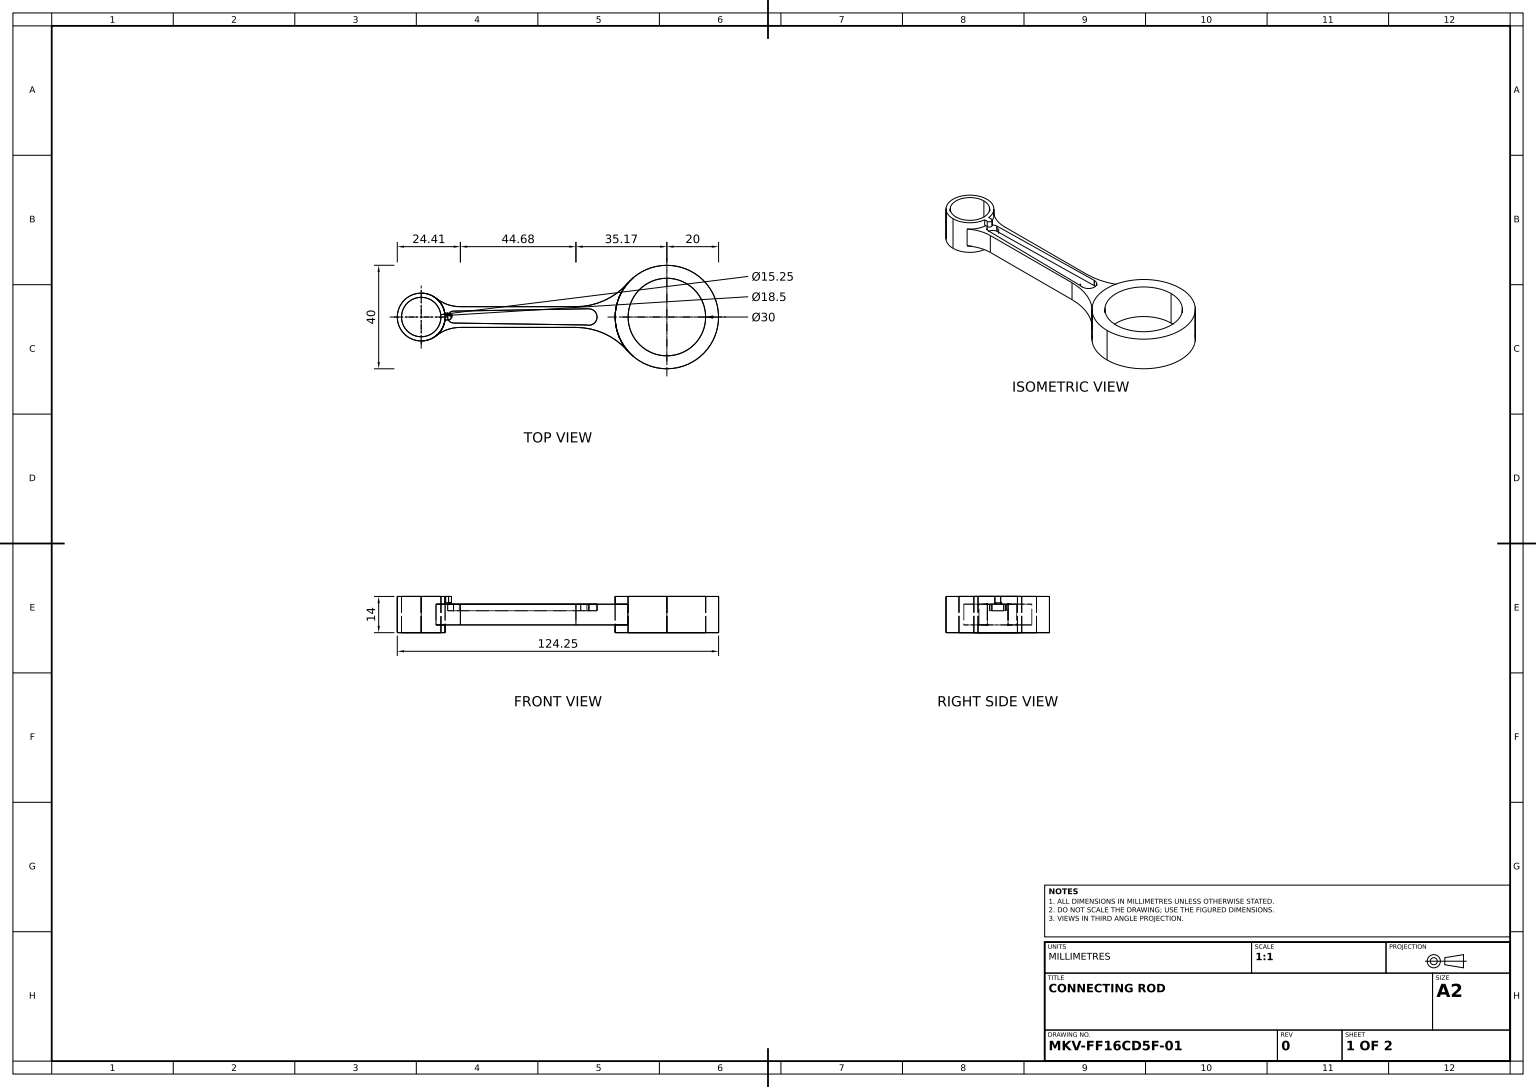
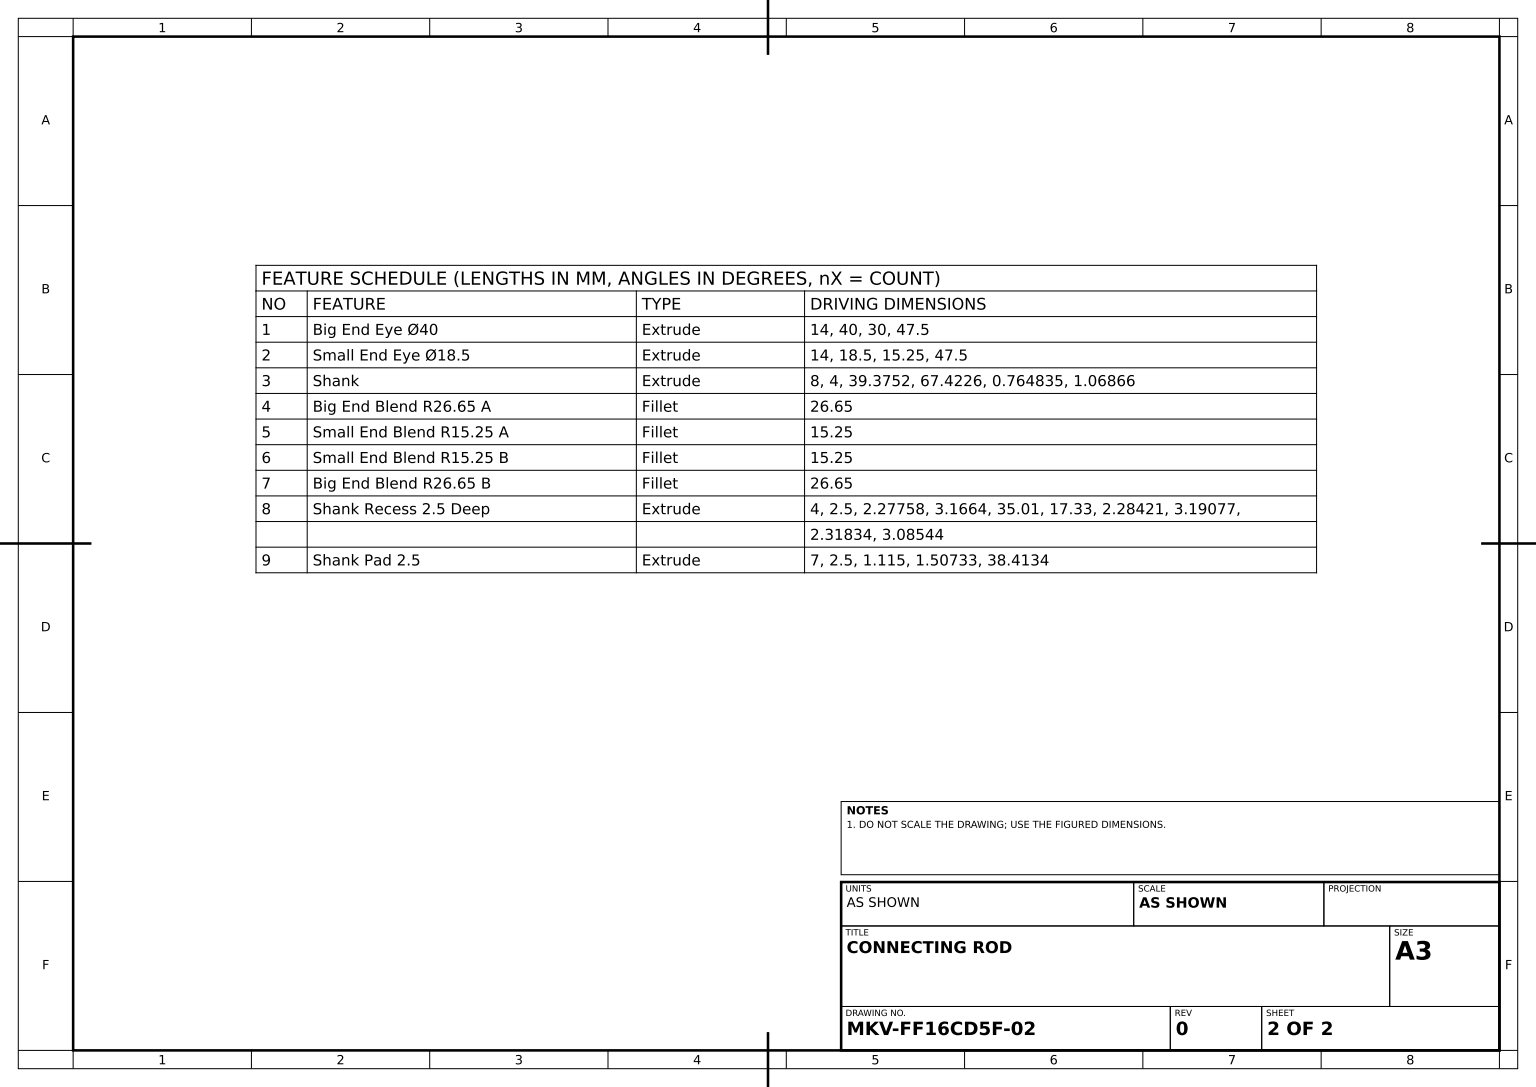
from build123d import *

# Parameters (mm, degrees)
BIG_END_EYE_SKETCH_R        = 20
BIG_END_EYE_SKETCH_R_2      = 15
BIG_END_EYE_40_DEPTH        = 7
SMALL_END_EYE_SKETCH_R      = 9.25
SMALL_END_EYE_SKETCH_R_2    = 7.625
SMALL_END_EYE_18_5_DEPTH    = 7
SHANK_DEPTH                 = 4
BIG_END_BLEND_R26_65_A_R    = 26.65
SMALL_END_BLEND_R15_25_A_R  = 15.25
SMALL_END_BLEND_R15_25_B_R  = 15.25
BIG_END_BLEND_R26_65_B_R    = 26.65
SHANK_RECESS_2_5_DEEP_DEPTH = 2.5
SHANK_PAD_2_5_DEPTH         = 2.5


with BuildPart() as part:
    # Big End Eye Sketch → Big End Eye Ø40 (new, symmetric)
    with BuildSketch(Plane(origin=(0, 0, 0), x_dir=(1, 0, 0), z_dir=(0, 1, 0))):
        with Locations(Location((47.5, 0, 0), (0, 0, 270))):
            Circle(BIG_END_EYE_SKETCH_R)
        with Locations(Location((47.5, 0, 0), (0, 0, 270))):
            Circle(BIG_END_EYE_SKETCH_R_2, mode=Mode.SUBTRACT)
    extrude(amount=BIG_END_EYE_40_DEPTH, both=True)



with BuildPart() as body_2:
    # Small End Eye Sketch → Small End Eye Ø18.5 (new, symmetric)
    with BuildSketch(Plane(origin=(0, 0, 0), x_dir=(1, 0, 0), z_dir=(0, 1, 0))):
        with Locations(Location((-47.5, 0, 0), (0, 0, 270))):
            Circle(SMALL_END_EYE_SKETCH_R)
        with Locations(Location((-47.5, 0, 0), (0, 0, 270))):
            Circle(SMALL_END_EYE_SKETCH_R_2, mode=Mode.SUBTRACT)
    extrude(amount=SMALL_END_EYE_18_5_DEPTH, both=True)


with BuildPart() as part_1:
    add(part.part)

    add(body_2.part)  # Shank merges body 2
    # Shank Profile Sketch → Shank (add, symmetric)
    with BuildSketch(Plane(origin=(0, 0, 0), x_dir=(1, 0, 0), z_dir=(0, 1, 0))):
        Polygon((27.282550476, 4), (28.047385708, 4), (28.047385708, -4), (-38.306518326, -4), (-39.375179325, -4), (-39.375179325, 4), align=None)
    extrude(amount=SHANK_DEPTH, both=True)

    # Big End Blend R26.65 A
    big_end_blend_r26_65_a_edges = [part_1.edges().sort_by_distance(p)[0] for p in [
        (27.904082058, 0, -4),
    ]]
    fillet(big_end_blend_r26_65_a_edges, radius=BIG_END_BLEND_R26_65_A_R)

    # Small End Blend R15.25 A
    small_end_blend_r15_25_a_edges = [part_1.edges().sort_by_distance(p)[0] for p in [
        (-39.159586341, 0, -4),
    ]]
    fillet(small_end_blend_r15_25_a_edges, radius=SMALL_END_BLEND_R15_25_A_R)

    # Small End Blend R15.25 B
    small_end_blend_r15_25_b_edges = [part_1.edges().sort_by_distance(p)[0] for p in [
        (-39.159586341, 0, 4),
    ]]
    fillet(small_end_blend_r15_25_b_edges, radius=SMALL_END_BLEND_R15_25_B_R)

    # Big End Blend R26.65 B
    big_end_blend_r26_65_b_edges = [part_1.edges().sort_by_distance(p)[0] for p in [
        (27.904082058, 0, 4),
    ]]
    fillet(big_end_blend_r26_65_b_edges, radius=BIG_END_BLEND_R26_65_B_R)

    # Shank Recess Sketch → Shank Recess 2.5 Deep (cut)
    with BuildSketch(Plane(origin=(0, 4, 0), x_dir=(1, 0, 0), z_dir=(0, 1, 0))):
        with BuildLine():
            ThreePointArc((-35.01, 2.277583754), (-37.287583754, 0), (-35.01, -2.277583754))
            Line((-35.01, -2.277583754), (-35.01, -2.318344298))
            Line((-35.01, -2.318344298), (16.571994255, -3.074327461))
            ThreePointArc((16.571994255, -3.074327461), (20.473294407, -0.381788318), (17.33, 3.16639575))
            Line((17.33, 3.16639575), (17.33, 3.190774264))
            Line((17.33, 3.190774264), (-35.01, 2.28421045))
            Line((-35.01, 2.28421045), (-35.01, 2.277583754))
        make_face()
    extrude(amount=-SHANK_RECESS_2_5_DEEP_DEPTH, mode=Mode.SUBTRACT)

    # Shank Pad Sketch → Shank Pad 2.5 (add)
    with BuildSketch(Plane(origin=(0, 7, 0), x_dir=(1, 0, 0), z_dir=(0, 1, 0))):
        with BuildLine():
            Line((-38.413384426, 0), (-36.90605517, 0))
            Line((-36.90605517, 0), (-35.79105517, 0))
            ThreePointArc((-35.79105517, 0), (-36.117631109, 0.788424061), (-36.90605517, 1.115))
            Line((-36.90605517, 1.115), (-38.413384426, 1.115))
            Line((-38.413384426, 1.115), (-38.413384426, 0))
        make_face()
        with BuildLine():
            Line((-35.79105517, 0), (-36.90605517, 0))
            Line((-36.90605517, 0), (-38.413384426, 0))
            Line((-38.413384426, 0), (-38.413384426, -1.115))
            Line((-38.413384426, -1.115), (-36.90605517, -1.115))
            ThreePointArc((-36.90605517, -1.115), (-36.117631109, -0.788424061), (-35.79105517, 0))
        make_face()
    extrude(amount=-SHANK_PAD_2_5_DEPTH)


solid = part_1.part
